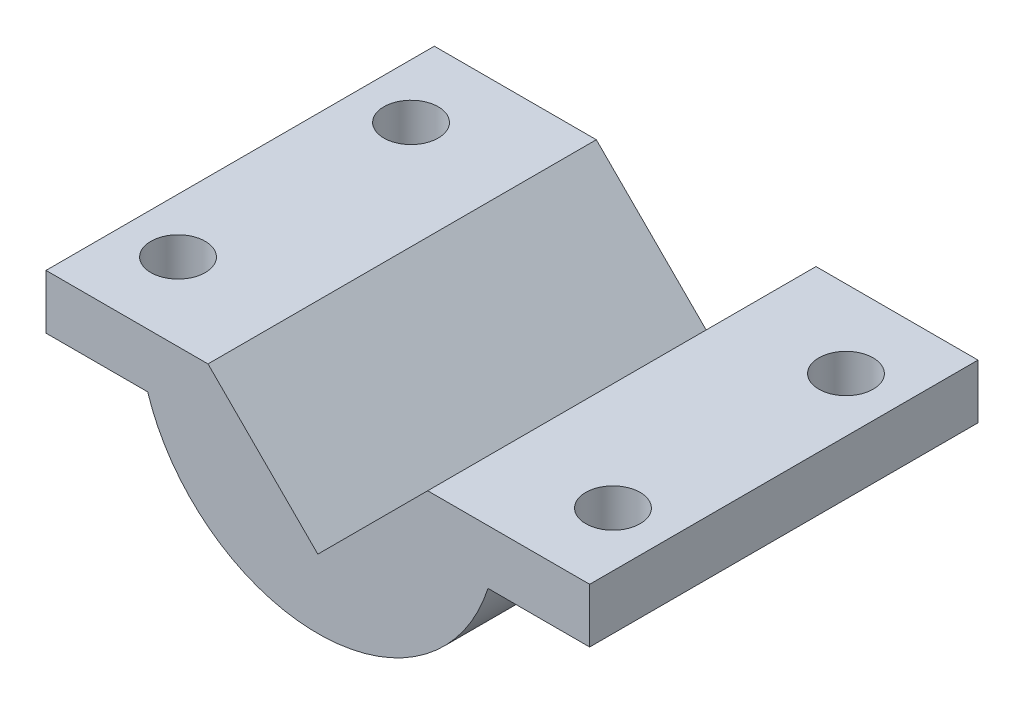
from build123d import *

# Parameters (mm, degrees)
SADDLE_BODY_DEPTH           = 25
FLANGE_MOUNTING_HOLES_REACH = 50.775
FLANGE_HOLES_SKETCH_R       = 3.5


with BuildPart() as part:
    # Saddle Profile Sketch → Saddle Body (new, symmetric)
    with BuildSketch(Plane.XY):
        with BuildLine():
            Line((0, -14.142135624), (14.142135624, 0))
            Line((14.142135624, 0), (35, 0))
            Line((35, 0), (35, -7))
            Line((35, -7), (21.9089023, -7))
            ThreePointArc((21.9089023, -7), (0, -23), (-21.9089023, -7))
            Line((-21.9089023, -7), (-35, -7))
            Line((-35, -7), (-35, 0))
            Line((-35, 0), (-14.142135624, 0))
            Line((-14.142135624, 0), (0, -14.142135624))
        make_face()
    extrude(amount=SADDLE_BODY_DEPTH, both=True)

    # Flange Holes Sketch → Flange Mounting Holes (cut, up to next)
    with BuildSketch(Plane(origin=(0, 0, 0), x_dir=(1, 0, 0), z_dir=(0, 1, 0)), mode=Mode.PRIVATE) as flange_mounting_holes_sk1:
        with Locations(Location((-28, 15, 0), (0, 0, 180))):
            Circle(FLANGE_HOLES_SKETCH_R)
    flange_mounting_holes_tool1 = extrude(flange_mounting_holes_sk1.sketch, amount=-FLANGE_MOUNTING_HOLES_REACH, mode=Mode.PRIVATE) & part.part
    # Flange Holes Sketch → Flange Mounting Holes (cut, up to next)
    with BuildSketch(Plane(origin=(0, 0, 0), x_dir=(1, 0, 0), z_dir=(0, 1, 0)), mode=Mode.PRIVATE) as flange_mounting_holes_sk2:
        with Locations(Location((-28, -15, 0), (0, 0, 180))):
            Circle(FLANGE_HOLES_SKETCH_R)
    flange_mounting_holes_tool2 = extrude(flange_mounting_holes_sk2.sketch, amount=-FLANGE_MOUNTING_HOLES_REACH, mode=Mode.PRIVATE) & part.part
    # Flange Holes Sketch → Flange Mounting Holes (cut, up to next)
    with BuildSketch(Plane(origin=(0, 0, 0), x_dir=(1, 0, 0), z_dir=(0, 1, 0)), mode=Mode.PRIVATE) as flange_mounting_holes_sk3:
        with Locations(Location((28, -15, 0), (0, 0, 180))):
            Circle(FLANGE_HOLES_SKETCH_R)
    flange_mounting_holes_tool3 = extrude(flange_mounting_holes_sk3.sketch, amount=-FLANGE_MOUNTING_HOLES_REACH, mode=Mode.PRIVATE) & part.part
    # Flange Holes Sketch → Flange Mounting Holes (cut, up to next)
    with BuildSketch(Plane(origin=(0, 0, 0), x_dir=(1, 0, 0), z_dir=(0, 1, 0)), mode=Mode.PRIVATE) as flange_mounting_holes_sk4:
        with Locations(Location((28, 15, 0), (0, 0, 180))):
            Circle(FLANGE_HOLES_SKETCH_R)
    flange_mounting_holes_tool4 = extrude(flange_mounting_holes_sk4.sketch, amount=-FLANGE_MOUNTING_HOLES_REACH, mode=Mode.PRIVATE) & part.part
    add(flange_mounting_holes_tool1.solids().sort_by_distance((-28, 0, -15))[0], mode=Mode.SUBTRACT)
    add(flange_mounting_holes_tool2.solids().sort_by_distance((-28, 0, 15))[0], mode=Mode.SUBTRACT)
    add(flange_mounting_holes_tool3.solids().sort_by_distance((28, 0, 15))[0], mode=Mode.SUBTRACT)
    add(flange_mounting_holes_tool4.solids().sort_by_distance((28, 0, -15))[0], mode=Mode.SUBTRACT)


solid = part.part
